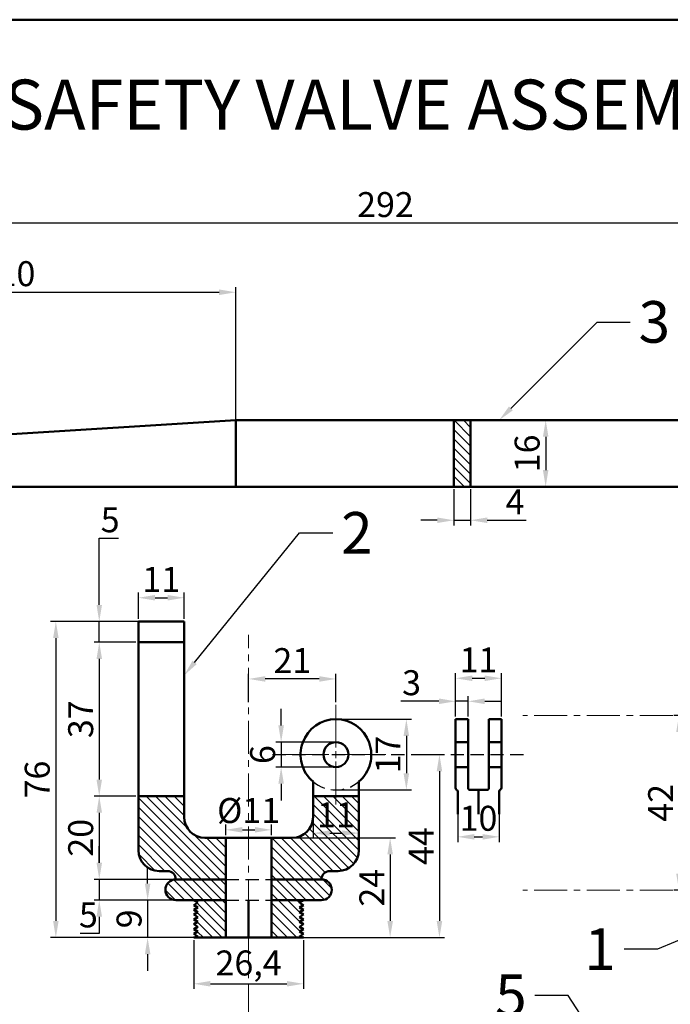
# Model space of a CAD drawing. Units: millimetres. Extents: x -25 to 763, y -62 to 306.
# Tile 6 of 7: x 440 to 597, y 69 to 306. Entities that reach past the tile are written whole.
import ezdxf
from ezdxf import colors
from ezdxf.entities.mleader import LeaderData, LeaderLine
from ezdxf.math import Vec2, Vec3

# ---------------------------------------------------------------- set-up
doc = ezdxf.new("R2010")
doc.units = ezdxf.units.MM
doc.header["$LTSCALE"] = 0.5
doc.linetypes.add('CENTER', pattern=[50.8, 31.75, -6.35, 6.35, -6.35])
doc.linetypes.add('DASHED', pattern=[19.05, 12.7, -6.35])
for name, color, linetype, lineweight in [('M-CNTR', 1, 'CENTER', 18), ('M-DIMS', 2, 'Continuous', 25), ('M-HATC', 8, 'Continuous', 18), ('M-HIDN', 4, 'DASHED', 25), ('M-OUTL', 7, 'Continuous', 50), ('M-TEXT', 3, 'Continuous', 25), ('M-TTLB', 7, 'Continuous', 50)]:
    doc.layers.add(name, color=color, linetype=linetype, lineweight=lineweight)
doc.styles.get("Standard").update_dxf_attribs({"font": 'arial.ttf'})
doc.dimstyles.new('ISO-25', dxfattribs={"dimtxt": 6, "dimasz": 4, "dimexe": 1.25, "dimexo": 0.625, "dimtad": 1, "dimtoh": 1, "dimdec": 1, "dimtxsty": 'Standard', "dimcen": 2.5, "dimadec": 0, "dimazin": 0, "dimtfac": 1, "dimtdec": 1, "dimtmove": 0, "dimatfit": 3, "dimfxl": 1, "dimarcsym": 0})

# ---------------------------------------------------------------- blocks, each defined once
blk = doc.blocks.new('*D22')
at = {"layer": 'Defpoints', "color": 0, "ltscale": 0.5, "transparency": 16777216}
for p in [(468.68, 161.08), (459.27, 156.08), (468.68, 156.08)]:
    blk.add_point(p, dxfattribs=at)
at = {"layer": 'M-DIMS', "color": 0, "lineweight": -2, "ltscale": 0.5, "transparency": 16777216}
for p, q in [((459.27, 165.08), (459.27, 181.08)), ((459.27, 181.08), (463.88, 181.08)), ((468.05, 161.08), (458.02, 161.08)), ((459.27, 156.08), (459.27, 161.08)), ((468.05, 156.08), (458.02, 156.08)), ((459.27, 152.08), (459.27, 148.08))]:
    blk.add_line(p, q, dxfattribs=at)
at = {"layer": 'M-DIMS', "color": 0, "ltscale": 0.5, "transparency": 16777216}
for points in [[(458.61, 165.08), (459.94, 165.08), (459.27, 161.08)], [(458.61, 152.08), (459.94, 152.08), (459.27, 156.08)]]:
    blk.add_solid(points, dxfattribs=at)
at = {"layer": 'M-DIMS', "color": 0, "ltscale": 0.5, "transparency": 16777216, "insert": (461.89, 184.75), "char_height": 6, "attachment_point": 5}
blk.add_mtext('5', dxfattribs=at)
blk = doc.blocks.new('*D23')
at = {"layer": 'Defpoints', "color": 0, "ltscale": 0.5, "transparency": 16777216}
for p in [(465.32, 156.08), (459.27, 119.08), (468.68, 119.08)]:
    blk.add_point(p, dxfattribs=at)
at = {"layer": 'M-DIMS', "color": 0, "lineweight": -2, "ltscale": 0.5, "transparency": 16777216}
for p, q in [((464.69, 156.08), (458.02, 156.08)), ((459.27, 152.08), (459.27, 123.08)), ((468.05, 119.08), (458.02, 119.08))]:
    blk.add_line(p, q, dxfattribs=at)
at = {"layer": 'M-DIMS', "color": 0, "ltscale": 0.5, "transparency": 16777216}
for points in [[(458.61, 152.08), (459.94, 152.08), (459.27, 156.08)], [(458.61, 123.08), (459.94, 123.08), (459.27, 119.08)]]:
    blk.add_solid(points, dxfattribs=at)
at = {"layer": 'M-DIMS', "color": 0, "ltscale": 0.5, "transparency": 16777216, "insert": (455.58, 137.58), "char_height": 6, "attachment_point": 5, "rotation": 90}
blk.add_mtext('37', dxfattribs=at)
blk = doc.blocks.new('*D24')
at = {"layer": 'Defpoints', "color": 0, "ltscale": 0.5, "transparency": 16777216}
for p in [(463.04, 119.08), (459.27, 99.08), (479.97, 99.08)]:
    blk.add_point(p, dxfattribs=at)
at = {"layer": 'M-DIMS', "color": 0, "lineweight": -2, "ltscale": 0.5, "transparency": 16777216}
for p, q in [((462.41, 119.08), (458.02, 119.08)), ((459.27, 115.08), (459.27, 103.08)), ((479.34, 99.08), (458.02, 99.08))]:
    blk.add_line(p, q, dxfattribs=at)
at = {"layer": 'M-DIMS', "color": 0, "ltscale": 0.5, "transparency": 16777216}
for points in [[(458.61, 115.08), (459.94, 115.08), (459.27, 119.08)], [(458.61, 103.08), (459.94, 103.08), (459.27, 99.08)]]:
    blk.add_solid(points, dxfattribs=at)
at = {"layer": 'M-DIMS', "color": 0, "ltscale": 0.5, "transparency": 16777216, "insert": (455.58, 109.08), "char_height": 6, "attachment_point": 5, "rotation": 90}
blk.add_mtext('20', dxfattribs=at)
blk = doc.blocks.new('*D25')
at = {"layer": 'Defpoints', "color": 0, "ltscale": 0.5, "transparency": 16777216}
for p in [(480.47, 99.08), (459.27, 94.08), (480.47, 94.08)]:
    blk.add_point(p, dxfattribs=at)
at = {"layer": 'M-DIMS', "color": 0, "lineweight": -2, "ltscale": 0.5, "transparency": 16777216}
for p, q in [((459.27, 103.08), (459.27, 107.08)), ((479.84, 99.08), (458.02, 99.08)), ((459.27, 99.08), (459.27, 94.08)), ((479.84, 94.08), (458.02, 94.08)), ((459.27, 90.08), (459.27, 86.08)), ((459.27, 86.08), (454.67, 86.08))]:
    blk.add_line(p, q, dxfattribs=at)
at = {"layer": 'M-DIMS', "color": 0, "ltscale": 0.5, "transparency": 16777216}
for points in [[(458.61, 103.08), (459.94, 103.08), (459.27, 99.08)], [(458.61, 90.08), (459.94, 90.08), (459.27, 94.08)]]:
    blk.add_solid(points, dxfattribs=at)
at = {"layer": 'M-DIMS', "color": 0, "ltscale": 0.5, "transparency": 16777216, "insert": (456.66, 89.76), "char_height": 6, "attachment_point": 5}
blk.add_mtext('5', dxfattribs=at)
blk = doc.blocks.new('*D26')
at = {"layer": 'Defpoints', "color": 0, "ltscale": 0.5, "transparency": 16777216}
for p in [(489.68, 94.08), (470.9, 85.08), (489.68, 85.08)]:
    blk.add_point(p, dxfattribs=at)
at = {"layer": 'M-DIMS', "color": 0, "lineweight": -2, "ltscale": 0.5, "transparency": 16777216}
for p, q in [((470.9, 98.08), (470.9, 102.08)), ((489.05, 94.08), (469.65, 94.08)), ((470.9, 94.08), (470.9, 85.08)), ((489.05, 85.08), (469.65, 85.08)), ((470.9, 81.08), (470.9, 77.08))]:
    blk.add_line(p, q, dxfattribs=at)
at = {"layer": 'M-DIMS', "color": 0, "ltscale": 0.5, "transparency": 16777216}
for points in [[(470.24, 98.08), (471.57, 98.08), (470.9, 94.08)], [(470.24, 81.08), (471.57, 81.08), (470.9, 85.08)]]:
    blk.add_solid(points, dxfattribs=at)
at = {"layer": 'M-DIMS', "color": 0, "ltscale": 0.5, "transparency": 16777216, "insert": (467.21, 89.58), "char_height": 6, "attachment_point": 5, "rotation": 90}
blk.add_mtext('9', dxfattribs=at)
blk = doc.blocks.new('*D27')
at = {"layer": 'Defpoints', "color": 0, "ltscale": 0.5, "transparency": 16777216}
for p in [(474.18, 161.08), (448.83, 85.08), (479.35, 85.08)]:
    blk.add_point(p, dxfattribs=at)
at = {"layer": 'M-DIMS', "color": 0, "lineweight": -2, "ltscale": 0.5, "transparency": 16777216}
for p, q in [((473.55, 161.08), (447.58, 161.08)), ((448.83, 157.08), (448.83, 89.08)), ((478.73, 85.08), (447.58, 85.08))]:
    blk.add_line(p, q, dxfattribs=at)
at = {"layer": 'M-DIMS', "color": 0, "ltscale": 0.5, "transparency": 16777216}
for points in [[(448.17, 157.08), (449.5, 157.08), (448.83, 161.08)], [(448.17, 89.08), (449.5, 89.08), (448.83, 85.08)]]:
    blk.add_solid(points, dxfattribs=at)
at = {"layer": 'M-DIMS', "color": 0, "ltscale": 0.5, "transparency": 16777216, "insert": (445.14, 123.08), "char_height": 6, "attachment_point": 5, "rotation": 90}
blk.add_mtext('76', dxfattribs=at)
blk = doc.blocks.new('*D28')
at = {"layer": 'Defpoints', "color": 0, "ltscale": 0.5, "transparency": 16777216}
for p in [(479.68, 166.78), (468.68, 161.08), (479.68, 161.08)]:
    blk.add_point(p, dxfattribs=at)
at = {"layer": 'M-DIMS', "color": 0, "lineweight": -2, "ltscale": 0.5, "transparency": 16777216}
for p, q in [((468.68, 161.7), (468.68, 168.03)), ((472.68, 166.78), (475.68, 166.78)), ((479.68, 161.7), (479.68, 168.03))]:
    blk.add_line(p, q, dxfattribs=at)
at = {"layer": 'M-DIMS', "color": 0, "ltscale": 0.5, "transparency": 16777216}
for points in [[(472.68, 167.45), (472.68, 166.12), (468.68, 166.78)], [(475.68, 167.45), (475.68, 166.12), (479.68, 166.78)]]:
    blk.add_solid(points, dxfattribs=at)
at = {"layer": 'M-DIMS', "color": 0, "ltscale": 0.5, "transparency": 16777216, "insert": (474.18, 170.42), "char_height": 6, "attachment_point": 5}
blk.add_mtext('11', dxfattribs=at)
blk = doc.blocks.new('*D29')
at = {"layer": 'Defpoints', "color": 0, "ltscale": 0.5, "transparency": 16777216}
for p in [(510.68, 114.08), (521.68, 114.34), (521.68, 110.2)]:
    blk.add_point(p, dxfattribs=at)
at = {"layer": 'M-DIMS', "color": 0, "lineweight": -2, "ltscale": 0.5, "transparency": 16777216}
for p, q in [((521.68, 113.71), (521.68, 108.95)), ((510.68, 113.45), (510.68, 108.95)), ((514.68, 110.2), (517.68, 110.2))]:
    blk.add_line(p, q, dxfattribs=at)
at = {"layer": 'M-DIMS', "color": 0, "ltscale": 0.5, "transparency": 16777216}
for points in [[(514.68, 110.86), (514.68, 109.53), (510.68, 110.2)], [(517.68, 110.86), (517.68, 109.53), (521.68, 110.2)]]:
    blk.add_solid(points, dxfattribs=at)
at = {"layer": 'M-DIMS', "color": 0, "ltscale": 0.5, "transparency": 16777216, "insert": (516.18, 113.83), "char_height": 6, "attachment_point": 5}
blk.add_mtext('11', dxfattribs=at)
blk = doc.blocks.new('*U30')
at = {"layer": 'M-CNTR', "color": 0, "transparency": 16777216}
for p, q in [((0, 1.7), (0, 12)), ((-12, 0), (-1.7, 0)), ((1.7, 0), (12, 0)), ((0, -12), (0, -1.7))]:
    blk.add_line(p, q, dxfattribs=at)
at = {"layer": 'M-CNTR', "color": 0, "linetype": 'Continuous', "transparency": 16777216}
for p, q in [((-0.85, 0), (0.85, 0)), ((0, -0.85), (0, 0.85))]:
    blk.add_line(p, q, dxfattribs=at)
blk = doc.blocks.new('*D31')
at = {"layer": 'Defpoints', "color": 0, "ltscale": 0.5, "transparency": 16777216}
for p in [(495.18, 147.26), (495.18, 141.08), (516.18, 141.08)]:
    blk.add_point(p, dxfattribs=at)
at = {"layer": 'M-DIMS', "color": 0, "lineweight": -2, "ltscale": 0.5, "transparency": 16777216}
for p, q in [((495.18, 141.7), (495.18, 148.51)), ((512.18, 147.26), (499.18, 147.26)), ((516.18, 141.7), (516.18, 148.51))]:
    blk.add_line(p, q, dxfattribs=at)
at = {"layer": 'M-DIMS', "color": 0, "ltscale": 0.5, "transparency": 16777216}
for points in [[(499.18, 147.93), (499.18, 146.6), (495.18, 147.26)], [(512.18, 147.93), (512.18, 146.6), (516.18, 147.26)]]:
    blk.add_solid(points, dxfattribs=at)
at = {"layer": 'M-DIMS', "color": 0, "ltscale": 0.5, "transparency": 16777216, "insert": (505.68, 150.9), "char_height": 6, "attachment_point": 5}
blk.add_mtext('21', dxfattribs=at)
blk = doc.blocks.new('*D32')
at = {"layer": 'Defpoints', "color": 0, "ltscale": 0.5, "transparency": 16777216}
for p in [(516.18, 132.08), (503, 126.08), (516.18, 126.08)]:
    blk.add_point(p, dxfattribs=at)
at = {"layer": 'M-DIMS', "color": 0, "lineweight": -2, "ltscale": 0.5, "transparency": 16777216}
for p, q in [((503, 136.08), (503, 140.08)), ((515.55, 132.08), (501.75, 132.08)), ((503, 132.08), (503, 126.08)), ((515.55, 126.08), (501.75, 126.08)), ((503, 122.08), (503, 118.08))]:
    blk.add_line(p, q, dxfattribs=at)
at = {"layer": 'M-DIMS', "color": 0, "ltscale": 0.5, "transparency": 16777216}
for points in [[(502.34, 136.08), (503.67, 136.08), (503, 132.08)], [(502.34, 122.08), (503.67, 122.08), (503, 126.08)]]:
    blk.add_solid(points, dxfattribs=at)
at = {"layer": 'M-DIMS', "color": 0, "ltscale": 0.5, "transparency": 16777216, "insert": (499.32, 129.08), "char_height": 6, "attachment_point": 5, "rotation": 90}
blk.add_mtext('6', dxfattribs=at)
blk = doc.blocks.new('*D33')
at = {"layer": 'Defpoints', "color": 0, "ltscale": 0.5, "transparency": 16777216}
for p in [(516.18, 137.58), (516.18, 120.58), (533.11, 120.58)]:
    blk.add_point(p, dxfattribs=at)
at = {"layer": 'M-DIMS', "color": 0, "lineweight": -2, "ltscale": 0.5, "transparency": 16777216}
for p, q in [((516.8, 137.58), (534.36, 137.58)), ((533.11, 133.58), (533.11, 124.58)), ((516.8, 120.58), (534.36, 120.58))]:
    blk.add_line(p, q, dxfattribs=at)
at = {"layer": 'M-DIMS', "color": 0, "ltscale": 0.5, "transparency": 16777216}
for points in [[(532.44, 133.58), (533.77, 133.58), (533.11, 137.58)], [(532.44, 124.58), (533.77, 124.58), (533.11, 120.58)]]:
    blk.add_solid(points, dxfattribs=at)
at = {"layer": 'M-DIMS', "color": 0, "ltscale": 0.5, "transparency": 16777216, "insert": (529.47, 129.08), "char_height": 6, "attachment_point": 5, "rotation": 90}
blk.add_mtext('17', dxfattribs=at)
blk = doc.blocks.new('*D34')
at = {"layer": 'Defpoints', "color": 0, "ltscale": 0.5, "transparency": 16777216}
for p in [(536, 129.08), (495.18, 85.08), (541.06, 85.08)]:
    blk.add_point(p, dxfattribs=at)
at = {"layer": 'M-DIMS', "color": 0, "lineweight": -2, "ltscale": 0.5, "transparency": 16777216}
for p, q in [((536.62, 129.08), (542.31, 129.08)), ((541.06, 125.08), (541.06, 89.08)), ((495.8, 85.08), (542.31, 85.08))]:
    blk.add_line(p, q, dxfattribs=at)
at = {"layer": 'M-DIMS', "color": 0, "ltscale": 0.5, "transparency": 16777216}
for points in [[(540.4, 125.08), (541.73, 125.08), (541.06, 129.08)], [(540.4, 89.08), (541.73, 89.08), (541.06, 85.08)]]:
    blk.add_solid(points, dxfattribs=at)
at = {"layer": 'M-DIMS', "color": 0, "ltscale": 0.5, "transparency": 16777216, "insert": (537.44, 107.08), "char_height": 6, "attachment_point": 5, "rotation": 90}
blk.add_mtext('44', dxfattribs=at)
blk = doc.blocks.new('*D35')
at = {"layer": 'Defpoints', "color": 0, "ltscale": 0.5, "transparency": 16777216}
for p in [(505.68, 109.08), (505.68, 85.08), (529.21, 85.08)]:
    blk.add_point(p, dxfattribs=at)
at = {"layer": 'M-DIMS', "color": 0, "lineweight": -2, "ltscale": 0.5, "transparency": 16777216}
for p, q in [((506.3, 109.08), (530.46, 109.08)), ((529.21, 105.08), (529.21, 89.08)), ((506.3, 85.08), (530.46, 85.08))]:
    blk.add_line(p, q, dxfattribs=at)
at = {"layer": 'M-DIMS', "color": 0, "ltscale": 0.5, "transparency": 16777216}
for points in [[(528.55, 105.08), (529.88, 105.08), (529.21, 109.08)], [(528.55, 89.08), (529.88, 89.08), (529.21, 85.08)]]:
    blk.add_solid(points, dxfattribs=at)
at = {"layer": 'M-DIMS', "color": 0, "ltscale": 0.5, "transparency": 16777216, "insert": (525.58, 97.08), "char_height": 6, "attachment_point": 5, "rotation": 90}
blk.add_mtext('24', dxfattribs=at)
blk = doc.blocks.new('*D36')
at = {"layer": 'Defpoints', "color": 0, "ltscale": 0.5, "transparency": 16777216}
for p in [(547.95, 141.89), (544.95, 137.58), (547.95, 137.58)]:
    blk.add_point(p, dxfattribs=at)
at = {"layer": 'M-DIMS', "color": 0, "lineweight": -2, "ltscale": 0.5, "transparency": 16777216}
for p, q in [((544.95, 138.2), (544.95, 143.14)), ((547.95, 138.2), (547.95, 143.14)), ((540.95, 141.89), (531.77, 141.89)), ((547.95, 141.89), (544.95, 141.89)), ((551.95, 141.89), (555.95, 141.89))]:
    blk.add_line(p, q, dxfattribs=at)
at = {"layer": 'M-DIMS', "color": 0, "ltscale": 0.5, "transparency": 16777216}
for points in [[(540.95, 142.56), (540.95, 141.23), (544.95, 141.89)], [(551.95, 142.56), (551.95, 141.23), (547.95, 141.89)]]:
    blk.add_solid(points, dxfattribs=at)
at = {"layer": 'M-DIMS', "color": 0, "ltscale": 0.5, "transparency": 16777216, "insert": (534.36, 145.58), "char_height": 6, "attachment_point": 5}
blk.add_mtext('3', dxfattribs=at)
blk = doc.blocks.new('*D37')
at = {"layer": 'Defpoints', "color": 0, "ltscale": 0.5, "transparency": 16777216}
for p in [(555.95, 147.42), (544.95, 137.58), (555.95, 137.58)]:
    blk.add_point(p, dxfattribs=at)
at = {"layer": 'M-DIMS', "color": 0, "lineweight": -2, "ltscale": 0.5, "transparency": 16777216}
for p, q in [((544.95, 138.2), (544.95, 148.67)), ((548.95, 147.42), (551.95, 147.42)), ((555.95, 138.2), (555.95, 148.67))]:
    blk.add_line(p, q, dxfattribs=at)
at = {"layer": 'M-DIMS', "color": 0, "ltscale": 0.5, "transparency": 16777216}
for points in [[(548.95, 148.09), (548.95, 146.76), (544.95, 147.42)], [(551.95, 148.09), (551.95, 146.76), (555.95, 147.42)]]:
    blk.add_solid(points, dxfattribs=at)
at = {"layer": 'M-DIMS', "color": 0, "ltscale": 0.5, "transparency": 16777216, "insert": (550.45, 151.06), "char_height": 6, "attachment_point": 5}
blk.add_mtext('11', dxfattribs=at)
blk = doc.blocks.new('*D38')
at = {"layer": 'Defpoints', "color": 0, "ltscale": 0.5, "transparency": 16777216}
for p in [(545.45, 117.5), (555.45, 117.5), (555.45, 109.31)]:
    blk.add_point(p, dxfattribs=at)
at = {"layer": 'M-DIMS', "color": 0, "lineweight": -2, "ltscale": 0.5, "transparency": 16777216}
for p, q in [((545.45, 116.88), (545.45, 108.06)), ((555.45, 116.88), (555.45, 108.06)), ((549.45, 109.31), (551.45, 109.31))]:
    blk.add_line(p, q, dxfattribs=at)
at = {"layer": 'M-DIMS', "color": 0, "ltscale": 0.5, "transparency": 16777216}
for points in [[(549.45, 109.97), (549.45, 108.64), (545.45, 109.31)], [(551.45, 109.97), (551.45, 108.64), (555.45, 109.31)]]:
    blk.add_solid(points, dxfattribs=at)
at = {"layer": 'M-DIMS', "color": 0, "ltscale": 0.5, "transparency": 16777216, "insert": (550.45, 112.99), "char_height": 6, "attachment_point": 5}
blk.add_mtext('10', dxfattribs=at)
blk = doc.blocks.new('*D39')
at = {"layer": 'Defpoints', "color": 0, "ltscale": 0.5, "transparency": 16777216}
for p in [(481.98, 85.08), (508.38, 85.08), (508.38, 73.98)]:
    blk.add_point(p, dxfattribs=at)
at = {"layer": 'M-DIMS', "color": 0, "lineweight": -2, "ltscale": 0.5, "transparency": 16777216}
for p, q in [((481.98, 84.45), (481.98, 72.73)), ((508.38, 84.45), (508.38, 72.73)), ((485.98, 73.98), (504.38, 73.98))]:
    blk.add_line(p, q, dxfattribs=at)
at = {"layer": 'M-DIMS', "color": 0, "ltscale": 0.5, "transparency": 16777216}
for points in [[(485.98, 74.65), (485.98, 73.32), (481.98, 73.98)], [(504.38, 74.65), (504.38, 73.32), (508.38, 73.98)]]:
    blk.add_solid(points, dxfattribs=at)
at = {"layer": 'M-DIMS', "color": 0, "ltscale": 0.5, "transparency": 16777216, "insert": (495.18, 78.21), "char_height": 6, "attachment_point": 5}
blk.add_mtext('26,4', dxfattribs=at)
blk = doc.blocks.new('*D40')
at = {"layer": 'Defpoints', "color": 0, "ltscale": 0.5, "transparency": 16777216}
for p in [(489.68, 109.08), (500.68, 110.99), (500.68, 109.08)]:
    blk.add_point(p, dxfattribs=at)
at = {"layer": 'M-DIMS', "color": 0, "lineweight": -2, "ltscale": 0.5, "transparency": 16777216}
for p, q in [((489.68, 109.7), (489.68, 112.24)), ((500.68, 109.7), (500.68, 112.24)), ((493.68, 110.99), (496.68, 110.99))]:
    blk.add_line(p, q, dxfattribs=at)
at = {"layer": 'M-DIMS', "color": 0, "ltscale": 0.5, "transparency": 16777216}
for points in [[(493.68, 111.66), (493.68, 110.33), (489.68, 110.99)], [(496.68, 111.66), (496.68, 110.33), (500.68, 110.99)]]:
    blk.add_solid(points, dxfattribs=at)
at = {"layer": 'M-DIMS', "color": 0, "ltscale": 0.5, "transparency": 16777216, "insert": (495.18, 114.85), "char_height": 6, "attachment_point": 5}
blk.add_mtext('%%C11', dxfattribs=at)
blk = doc.blocks.new('*D62')
at = {"layer": 'Defpoints', "color": 0, "ltscale": 0.5, "transparency": 16777216}
for p in [(492.09, 240.22), (382.09, 194.54), (492.09, 194.54)]:
    blk.add_point(p, dxfattribs=at)
at = {"layer": 'M-DIMS', "color": 0, "lineweight": -2, "ltscale": 0.5, "transparency": 16777216}
for p, q in [((382.09, 195.17), (382.09, 241.47)), ((492.09, 195.17), (492.09, 241.47)), ((386.09, 240.22), (488.09, 240.22))]:
    blk.add_line(p, q, dxfattribs=at)
at = {"layer": 'M-DIMS', "color": 0, "ltscale": 0.5, "transparency": 16777216}
for points in [[(386.09, 240.89), (386.09, 239.55), (382.09, 240.22)], [(488.09, 240.89), (488.09, 239.55), (492.09, 240.22)]]:
    blk.add_solid(points, dxfattribs=at)
at = {"layer": 'M-DIMS', "color": 0, "ltscale": 0.5, "transparency": 16777216, "insert": (437.09, 243.91), "char_height": 6, "attachment_point": 5}
blk.add_mtext('110', dxfattribs=at)
blk = doc.blocks.new('*D67')
at = {"layer": 'Defpoints', "color": 0, "ltscale": 0.5, "transparency": 16777216}
for p in [(382.09, 256.83), (674.09, 201.48), (382.09, 197.48)]:
    blk.add_point(p, dxfattribs=at)
at = {"layer": 'M-DIMS', "color": 0, "lineweight": -2, "ltscale": 0.5, "transparency": 16777216}
for p, q in [((382.09, 198.1), (382.09, 258.08)), ((674.09, 202.1), (674.09, 258.08)), ((670.09, 256.83), (386.09, 256.83))]:
    blk.add_line(p, q, dxfattribs=at)
at = {"layer": 'M-DIMS', "color": 0, "ltscale": 0.5, "transparency": 16777216}
for points in [[(386.09, 257.5), (386.09, 256.17), (382.09, 256.83)], [(670.09, 257.5), (670.09, 256.17), (674.09, 256.83)]]:
    blk.add_solid(points, dxfattribs=at)
at = {"layer": 'M-DIMS', "color": 0, "ltscale": 0.5, "transparency": 16777216, "insert": (528.09, 260.52), "char_height": 6, "attachment_point": 5}
blk.add_mtext('292', dxfattribs=at)
blk = doc.blocks.new('*D68')
at = {"layer": 'Defpoints', "color": 0, "ltscale": 0.5, "transparency": 16777216}
for p in [(544.55, 193.48), (548.55, 193.48), (548.55, 185.41)]:
    blk.add_point(p, dxfattribs=at)
at = {"layer": 'M-DIMS', "color": 0, "lineweight": -2, "ltscale": 0.5, "transparency": 16777216}
for p, q in [((544.55, 192.85), (544.55, 184.16)), ((548.55, 192.85), (548.55, 184.16)), ((540.55, 185.41), (536.55, 185.41)), ((544.55, 185.41), (548.55, 185.41)), ((552.55, 185.41), (561.95, 185.41))]:
    blk.add_line(p, q, dxfattribs=at)
at = {"layer": 'M-DIMS', "color": 0, "ltscale": 0.5, "transparency": 16777216}
for points in [[(540.55, 186.08), (540.55, 184.75), (544.55, 185.41)], [(552.55, 186.08), (552.55, 184.75), (548.55, 185.41)]]:
    blk.add_solid(points, dxfattribs=at)
at = {"layer": 'M-DIMS', "color": 0, "ltscale": 0.5, "transparency": 16777216, "insert": (559.25, 189.04), "char_height": 6, "attachment_point": 5}
blk.add_mtext('4', dxfattribs=at)
blk = doc.blocks.new('*D69')
at = {"layer": 'Defpoints', "color": 0, "ltscale": 0.5, "transparency": 16777216}
for p in [(555.43, 209.48), (555.43, 193.48), (566.61, 193.48)]:
    blk.add_point(p, dxfattribs=at)
at = {"layer": 'M-DIMS', "color": 0, "lineweight": -2, "ltscale": 0.5, "transparency": 16777216}
for p, q in [((556.05, 209.48), (567.86, 209.48)), ((566.61, 205.48), (566.61, 197.48)), ((556.05, 193.48), (567.86, 193.48))]:
    blk.add_line(p, q, dxfattribs=at)
at = {"layer": 'M-DIMS', "color": 0, "ltscale": 0.5, "transparency": 16777216}
for points in [[(565.94, 205.48), (567.27, 205.48), (566.61, 209.48)], [(565.94, 197.48), (567.27, 197.48), (566.61, 193.48)]]:
    blk.add_solid(points, dxfattribs=at)
at = {"layer": 'M-DIMS', "color": 0, "ltscale": 0.5, "transparency": 16777216, "insert": (562.92, 201.48), "char_height": 6, "attachment_point": 5, "rotation": 90}
blk.add_mtext('16', dxfattribs=at)
blk = doc.blocks.new('*D78')
at = {"layer": 'Defpoints', "color": 0, "ltscale": 0.5, "transparency": 16777216}
for p in [(598.66, 138.48), (608.6, 138.48), (653.09, 96.48)]:
    blk.add_point(p, dxfattribs=at)
at = {"layer": 'M-DIMS', "color": 0, "lineweight": -2, "ltscale": 0.5, "transparency": 16777216}
for p, q in [((607.98, 138.48), (597.41, 138.48)), ((598.66, 100.48), (598.66, 134.48)), ((652.47, 96.48), (597.41, 96.48))]:
    blk.add_line(p, q, dxfattribs=at)
at = {"layer": 'M-DIMS', "color": 0, "ltscale": 0.5, "transparency": 16777216}
for points in [[(597.99, 134.48), (599.32, 134.48), (598.66, 138.48)], [(597.99, 100.48), (599.32, 100.48), (598.66, 96.48)]]:
    blk.add_solid(points, dxfattribs=at)
at = {"layer": 'M-DIMS', "color": 0, "ltscale": 0.5, "transparency": 16777216, "insert": (595.02, 117.48), "char_height": 6, "attachment_point": 5, "rotation": 90}
blk.add_mtext('42', dxfattribs=at)

msp = doc.modelspace()

# ---------------------------------------------------------------- hatches: boundary and pattern name
at = {"layer": 'M-HATC', "ltscale": 0.5}
h = msp.add_hatch(dxfattribs=at)
h.set_pattern_fill('ANSI31', color=256, scale=0.5, angle=90)
h.set_pattern_definition([(135, (-6.016, -7.7459), (-1.122532, -1.122532), [])])
h.paths.add_polyline_path([(544.55, 193.48), (548.55, 193.48), (548.55, 209.48), (544.55, 209.48)])
h = msp.add_hatch(dxfattribs=at)
h.set_pattern_fill('ANSI31', color=256, scale=0.5, angle=90)
h.set_pattern_definition([(135, (-56.0338, -32.3511), (-1.122532, -1.122532), [])])
h.paths.add_polyline_path([(489.68, 109.08), (484.68, 109.08, -0.414214), (479.68, 114.08), (479.68, 119.08), (468.68, 119.08), (468.68, 106.08, 0.414214), (473.68, 101.08), (475.68, 101.08, -0.414214), (477.68, 99.08), (481.46, 99.08), (489.68, 99.08)])
h.paths.add_polyline_path([(489.68, 85.08), (481.98, 85.08), (482.98, 85.38), (481.98, 85.96), (482.98, 86.54), (481.98, 87.13), (482.98, 87.7), (481.98, 88.28), (482.98, 88.86), (481.98, 89.43), (482.98, 90.01), (481.98, 90.6), (482.98, 91.18), (481.98, 91.76), (482.98, 92.33), (481.98, 92.91), (482.98, 93.49), (481.98, 94.08), (489.68, 94.08)])
h.paths.add_polyline_path([(489.68, 99.08), (481.46, 99.08), (477.68, 99.08, 1), (477.68, 94.08), (489.68, 94.08)])
h.paths.add_polyline_path([(521.68, 106.08), (521.68, 119.08), (510.68, 119.08), (510.68, 114.08, -0.414214), (505.68, 109.08), (500.68, 109.08), (500.68, 99.08), (512.68, 99.08, -0.414214), (514.68, 101.08), (516.68, 101.08, 0.414214)])
h.paths.add_polyline_path([(512.68, 99.08), (500.68, 99.08), (500.68, 94.08), (512.68, 94.08, 1)])
h.paths.add_polyline_path([(508.38, 94.08), (500.68, 94.08), (500.68, 85.08), (508.38, 85.08), (507.38, 85.38), (508.38, 85.96), (507.38, 86.54), (508.38, 87.13), (507.38, 87.7), (508.38, 88.28), (507.38, 88.86), (508.38, 89.43), (507.38, 90.01), (508.38, 90.6), (507.38, 91.18), (508.38, 91.76), (507.38, 92.33), (508.38, 92.91), (507.38, 93.49)])
h.paths.add_polyline_path([(522.18, 39.2), (508.38, 39.2), (508.38, 34.2), (522.18, 34.2)])
h.paths.add_polyline_path([(522.18, 34.2), (508.38, 34.2), (508.38, 29.2), (522.18, 29.2)])
h.paths.add_polyline_path([(481.98, 39.2), (468.18, 39.2), (468.18, 34.2), (481.98, 34.2)])
h.paths.add_polyline_path([(481.98, 34.2), (468.18, 34.2), (468.18, 29.2), (481.98, 29.2)])

# ---------------------------------------------------------------- linework, layer by layer
at = {"layer": 'M-CNTR', "ltscale": 0.5}
for p, q in [((495.18, -10.41), (495.18, 157.83)), ((749.56, 138.48), (561.14, 138.48)), ((749.56, 96.48), (561.14, 96.48))]:
    msp.add_line(p, q, dxfattribs=at)
at = {"layer": 'M-HIDN', "ltscale": 0.5}
for p, q in [((500.92, 129.08), (561.53, 129.08)), ((489.68, 99.08), (500.68, 99.08)), ((489.68, 94.08), (500.68, 94.08))]:
    msp.add_line(p, q, dxfattribs=at)
msp.add_arc((516.18, 129.08), 8.5, 229.6798, 310.3202, dxfattribs=at)
at = {"layer": 'M-OUTL', "ltscale": 0.5}
for p, q in [((395.09, 203.48), (492.09, 209.48)), ((492.09, 201.48), (492.09, 209.48)), ((492.09, 209.48), (626.59, 209.48)), ((544.55, 209.48), (544.55, 193.48)), ((548.55, 209.48), (548.55, 193.48)), ((492.09, 193.48), (492.09, 201.48)), ((626.59, 193.48), (382.09, 193.48)), ((479.68, 161.08), (468.68, 161.08)), ((468.68, 161.08), (468.68, 119.08)), ((479.68, 161.08), (479.68, 114.08)), ((479.68, 156.08), (468.68, 156.08)), ((544.95, 137.58), (544.95, 121.08)), ((544.95, 137.58), (547.95, 137.58)), ((547.95, 137.58), (547.95, 121.08)), ((552.95, 137.58), (552.95, 121.08)), ((555.95, 137.58), (552.95, 137.58)), ((555.95, 121.08), (555.95, 137.58)), ((544.95, 132.08), (547.95, 132.08)), ((552.95, 132.08), (555.95, 132.08)), ((544.95, 126.08), (547.95, 126.08)), ((552.95, 126.08), (555.95, 126.08)), ((510.68, 122.6), (510.68, 114.08)), ((521.68, 122.6), (521.68, 106.08)), ((468.68, 119.08), (479.68, 119.08)), ((468.68, 119.08), (468.68, 106.08)), ((510.68, 119.08), (521.68, 119.08)), ((545.45, 120.58), (545.45, 120.58)), ((545.45, 120.21), (545.45, 114.79)), ((548.45, 120.58), (552.45, 120.58)), ((550.45, 120.58), (550.45, 114.79)), ((555.45, 120.58), (555.45, 120.58)), ((555.45, 120.21), (555.45, 114.79)), ((484.68, 109.08), (505.68, 109.08)), ((489.68, 109.08), (489.68, 85.08)), ((500.68, 109.08), (500.68, 85.08)), ((475.68, 101.08), (473.68, 101.08)), ((514.68, 101.08), (516.68, 101.08)), ((477.68, 99.08), (489.68, 99.08)), ((481.46, 99.08), (477.68, 99.08)), ((477.68, 99.08), (477.68, 99.08)), ((500.68, 99.08), (512.68, 99.08)), ((512.68, 99.08), (512.68, 99.08)), ((477.68, 94.08), (489.68, 94.08)), ((495.18, 94.08), (495.18, 85.08)), ((500.68, 94.08), (512.68, 94.08)), ((481.98, 85.08), (482.98, 85.38)), ((508.38, 85.08), (507.38, 85.38)), ((481.98, 85.08), (508.38, 85.08))]:
    msp.add_line(p, q, dxfattribs=at)
at = {"layer": 'M-OUTL'}
for p, q in [((482.98, 93.49), (481.98, 92.91)), ((481.98, 92.91), (482.98, 92.33)), ((482.98, 92.33), (481.98, 91.76)), ((482.1, 94.01), (482.98, 93.49)), ((508.26, 94.01), (507.38, 93.49)), ((507.38, 93.49), (508.38, 92.91)), ((508.38, 92.91), (507.38, 92.33)), ((507.38, 92.33), (508.38, 91.76)), ((481.98, 91.76), (482.98, 91.18)), ((482.98, 91.18), (481.98, 90.6)), ((481.98, 90.6), (482.98, 90.01)), ((482.98, 90.01), (481.98, 89.43)), ((508.38, 91.76), (507.38, 91.18)), ((507.38, 91.18), (508.38, 90.6)), ((508.38, 90.6), (507.38, 90.01)), ((507.38, 90.01), (508.38, 89.43)), ((481.98, 89.43), (482.98, 88.86)), ((482.98, 88.86), (481.98, 88.28)), ((481.98, 88.28), (482.98, 87.7)), ((482.98, 87.7), (481.98, 87.13)), ((508.38, 89.43), (507.38, 88.86)), ((507.38, 88.86), (508.38, 88.28)), ((508.38, 88.28), (507.38, 87.7)), ((507.38, 87.7), (508.38, 87.13)), ((481.98, 87.13), (482.98, 86.54)), ((482.98, 86.54), (481.98, 85.96)), ((481.98, 85.96), (482.98, 85.38)), ((508.38, 87.13), (507.38, 86.54)), ((507.38, 86.54), (508.38, 85.96)), ((508.38, 85.96), (507.38, 85.38))]:
    msp.add_line(p, q, dxfattribs=at)
at = {"layer": 'M-OUTL', "ltscale": 0.5}
msp.add_circle((516.18, 129.08), 3, dxfattribs=at)
for centre, radius, start, end in [((516.18, 129.08), 8.5, 310.3202, 229.6798), ((545.45, 121.08), 0.5, 180, 240), ((548.45, 121.08), 0.5, 180, 270), ((552.45, 121.08), 0.5, 270, 0), ((555.45, 121.08), 0.5, 300, 360), ((544.95, 120.21), 0.5, 0, 60), ((555.95, 120.21), 0.5, 120, 180), ((484.68, 114.08), 5, 180, 270), ((505.68, 114.08), 5, 270, 0), ((473.68, 106.08), 5, 180, 270), ((516.68, 106.08), 5, 270, 360), ((475.68, 99.08), 2, 360, 90), ((514.68, 99.08), 2, 90, 180), ((477.68, 96.58), 2.5, 90, 270), ((512.68, 96.58), 2.5, 270, 90)]:
    msp.add_arc(centre, radius, start, end, dxfattribs=at)
at = {"layer": 'M-TTLB', "ltscale": 0.5}
msp.add_lwpolyline([(229.22, 305.74), (763.29, 305.74), (763.29, -62.45), (229.22, -62.45)], close=True, dxfattribs=at)

# ---------------------------------------------------------------- block references
at = {"layer": 'M-CNTR'}
msp.add_blockref('*U30', (516.18, 129.08), dxfattribs=at)

# ---------------------------------------------------------------- texts
at = {"layer": 'M-TTLB', "ltscale": 0.5, "insert": (403.69, 291.33), "char_height": 12, "attachment_point": 1}
msp.add_mtext_dynamic_manual_height_columns('\\pxqc;SAFETY VALVE ASSEMBLY', width=257.4414, gutter_width=12.5, heights=[0], dxfattribs=at)

# ---------------------------------------------------------------- dimensions: what is measured, and where the dimension line sits
at = {"layer": 'M-DIMS', "ltscale": 0.5}
for base, p1, p2, picture, middle in [((382.09, 256.83), (674.09, 201.48), (382.09, 197.48), '*D67', (528.09, 260.52)), ((492.09, 240.22), (382.09, 194.54), (492.09, 194.54), '*D62', (437.09, 243.91)), ((548.55, 185.41), (544.55, 193.48), (548.55, 193.48), '*D68', (559.25, 189.04)), ((479.68, 166.78), (468.68, 161.08), (479.68, 161.08), '*D28', (474.18, 170.42)), ((495.18, 147.26), (516.18, 141.08), (495.18, 141.08), '*D31', (505.68, 150.9)), ((521.68, 110.2), (510.68, 114.08), (521.68, 114.34), '*D29', (516.18, 113.83)), ((555.45, 109.31), (545.45, 117.5), (555.45, 117.5), '*D38', (550.45, 112.99)), ((508.38, 73.98), (481.98, 85.08), (508.38, 85.08), '*D39', (495.18, 78.21))]:
    dim = msp.add_linear_dim(base=base, p1=p1, p2=p2, dimstyle='ISO-25', override={"dimclrd": 0, "dimclre": 0, "dimclrt": 0}, dxfattribs=at)
    dim.commit()
    dim.dimension.update_dxf_attribs({"geometry": picture, "text_midpoint": middle})
for base, p1, p2, picture, middle in [((566.61, 193.48), (555.43, 209.48), (555.43, 193.48), '*D69', (562.92, 201.48)), ((459.27, 119.08), (465.32, 156.08), (468.68, 119.08), '*D23', (455.58, 137.58)), ((503, 126.08), (516.18, 132.08), (516.18, 126.08), '*D32', (499.32, 129.08)), ((533.11, 120.58), (516.18, 137.58), (516.18, 120.58), '*D33', (529.47, 129.08)), ((598.66, 138.48), (653.09, 96.48), (608.6, 138.48), '*D78', (595.02, 117.48)), ((541.06, 85.08), (536, 129.08), (495.18, 85.08), '*D34', (537.44, 107.08)), ((459.27, 99.08), (463.04, 119.08), (479.97, 99.08), '*D24', (455.58, 109.08)), ((529.21, 85.08), (505.68, 109.08), (505.68, 85.08), '*D35', (525.58, 97.08)), ((459.27, 94.08), (480.47, 99.08), (480.47, 94.08), '*D25', (456.66, 89.76)), ((470.9, 85.08), (489.68, 94.08), (489.68, 85.08), '*D26', (467.21, 89.58))]:
    dim = msp.add_linear_dim(base=base, p1=p1, p2=p2, angle=90, dimstyle='ISO-25', override={"dimclrd": 0, "dimclre": 0, "dimclrt": 0}, dxfattribs=at)
    dim.commit()
    dim.dimension.update_dxf_attribs({"geometry": picture, "text_midpoint": middle})
for base, p1, p2, picture, middle in [((459.27, 156.08), (468.68, 161.08), (468.68, 156.08), '*D22', (461.89, 181.08)), ((448.83, 85.08), (474.18, 161.08), (479.35, 85.08), '*D27', (448.83, 123.08))]:
    dim = msp.add_linear_dim(base=base, p1=p1, p2=p2, angle=90, dimstyle='ISO-25', override={"dimclrd": 0, "dimclre": 0, "dimclrt": 0}, dxfattribs=at)
    dim.commit()
    dim.dimension.update_dxf_attribs({"geometry": picture, "text_midpoint": middle, "dimtype": 160})
for base, p2, picture, middle in [((555.95, 147.42), (555.95, 137.58), '*D37', (550.45, 147.42)), ((547.95, 141.89), (547.95, 137.58), '*D36', (534.36, 141.89))]:
    dim = msp.add_linear_dim(base=base, p1=(544.95, 137.58), p2=p2, dimstyle='ISO-25', override={"dimclrd": 0, "dimclre": 0, "dimclrt": 0}, dxfattribs=at)
    dim.commit()
    dim.dimension.update_dxf_attribs({"geometry": picture, "text_midpoint": middle, "dimtype": 160})
dim = msp.add_linear_dim(base=(500.68, 110.99), p1=(489.68, 109.08), p2=(500.68, 109.08), text='%%C<>', dimstyle='ISO-25', override={"dimclrd": 0, "dimclre": 0, "dimclrt": 0}, dxfattribs=at)
dim.commit()
dim.dimension.update_dxf_attribs({"geometry": '*D40', "text_midpoint": (495.18, 110.99), "dimtype": 160})

# ---------------------------------------------------------------- leaders
at = {"layer": 'M-TEXT', "ltscale": 0.5}
ml = msp.add_multileader_mtext('Standard', dxfattribs=at)
ml.set_content('3', color=256)
ml.set_leader_properties()
ml.build(insert=Vec2(0, 0))
ctx = ml.context
ctx.base_point, ctx.char_height, ctx.plane_origin = Vec3(586.95, 233), 10, Vec3(555.43, 209.48)
notes = []
notes.append((ctx, [(0, (1, 1, 0), (578.95, 233), (1, 0), 8, [(0, [(555.43, 209.48)], 0, [])])]))
ctx.mtext.insert, ctx.mtext.flow_direction = Vec3(588.95, 238.09), 5
ml = msp.add_multileader_mtext('Standard', dxfattribs=at)
ml.set_content('2', color=256)
ml.set_leader_properties()
ml.build(insert=Vec2(0, 0))
ctx = ml.context
ctx.base_point, ctx.char_height, ctx.plane_origin = Vec3(515.42, 182.39), 10, Vec3(479.68, 148.13)
notes.append((ctx, [(0, (1, 1, 0), (507.42, 182.39), (1, 0), 8, [(0, [(479.68, 148.13)], 0, [])])]))
ctx.mtext.insert, ctx.mtext.flow_direction = Vec3(517.42, 187.39), 5
ml = msp.add_multileader_mtext('Standard', dxfattribs=at)
ml.set_content('1', color=256)
ml.set_leader_properties()
ml.build(insert=Vec2(0, 0))
ctx = ml.context
ctx.base_point, ctx.char_height, ctx.plane_origin = Vec3(577.79, 82.32), 10, Vec3(632.11, 98.48)
ctx.text_align_type = 2
notes.append((ctx, [(0, (1, 1, 0), (593.48, 82.32), (-1, 0), 8, [(0, [(632.11, 98.48)], 0, [])])]))
ctx.mtext.insert, ctx.mtext.alignment, ctx.mtext.flow_direction = Vec3(583.48, 87.32), 3, 5
ml = msp.add_multileader_mtext('Standard', dxfattribs=at)
ml.set_content('5', color=256)
ml.set_leader_properties()
ml.build(insert=Vec2(0, 0))
ctx = ml.context
ctx.base_point, ctx.char_height, ctx.plane_origin = Vec3(553.41, 71.15), 10, Vec3(583.59, 53.42)
ctx.text_align_type = 2
notes.append((ctx, [(0, (1, 1, 0), (572.04, 71.15), (-1, 0), 8, [(0, [(583.59, 53.42)], 0, [])])]))
ctx.mtext.insert, ctx.mtext.alignment, ctx.mtext.flow_direction = Vec3(562.04, 76.23), 3, 5
for ctx, leaders in notes:
    for number, flags, end, landing, length, lines in leaders:
        leader = LeaderData()
        leader.index, (leader.has_last_leader_line, leader.has_dogleg_vector, leader.attachment_direction) = number, flags
        leader.last_leader_point, leader.dogleg_vector, leader.dogleg_length = Vec3(end), Vec3(landing), length
        for number, points, colour, breaks in lines:
            line = LeaderLine()
            line.index, line.vertices, line.color, line.breaks = number, Vec3.list(points), colors.encode_raw_color(colour), breaks
            leader.lines.append(line)
        ctx.leaders.append(leader)

doc.saveas('drawing.dxf')
